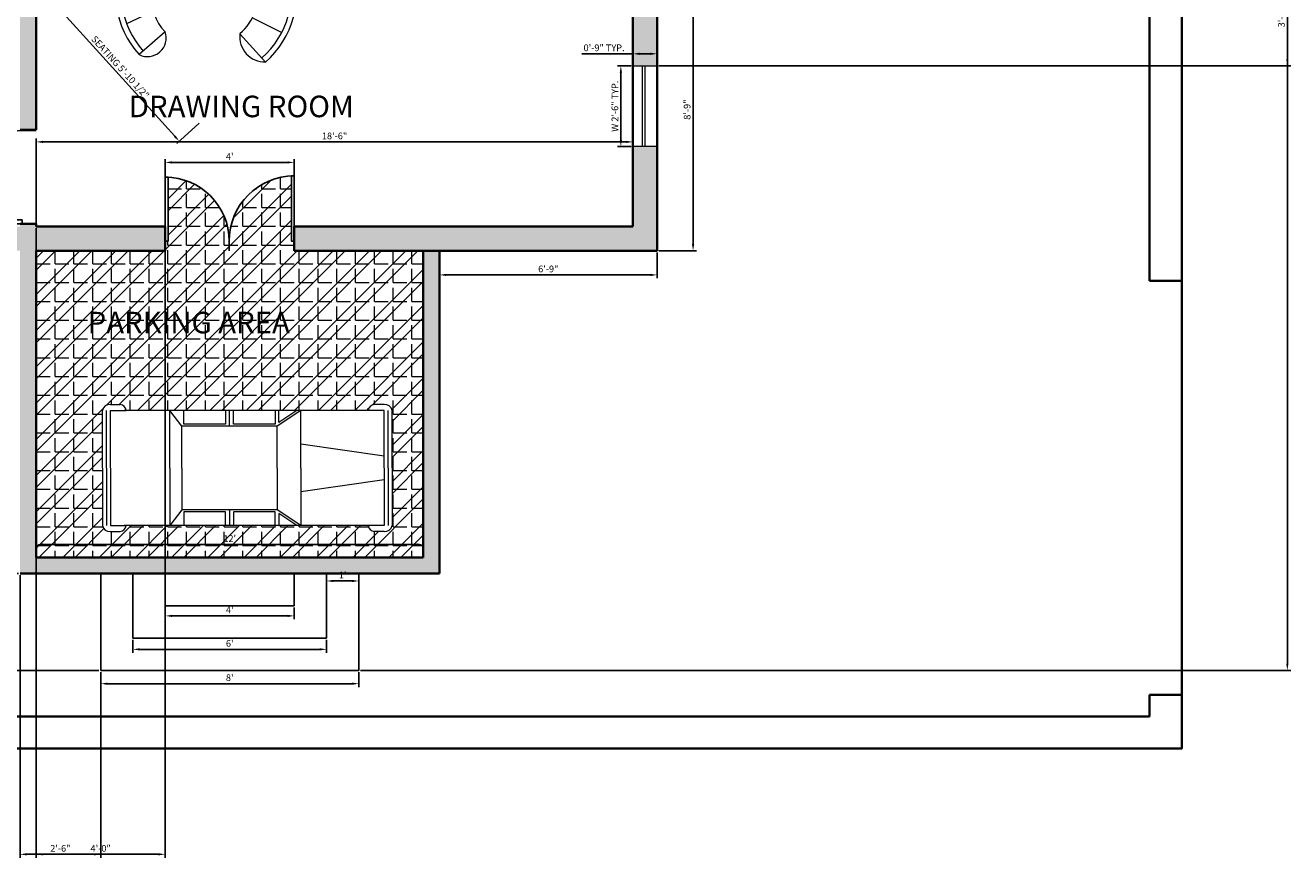
# Model space of a CAD drawing. Units: inches. Extents: x 2901 to 5923, y 918 to 2827.
# Tile 9 of 16: x 4585 to 5056, y 918 to 1227. Entities that reach past the tile are written whole.
import ezdxf

# ---------------------------------------------------------------- set-up
doc = ezdxf.new("R2010")
doc.units = ezdxf.units.IN
for name, color, linetype, lineweight in [('A-ANNO-DIMS', 2, 'Continuous', 18), ('A-AREA-IDEN', 7, 'Continuous', 25), ('A-EQPM-VEHI', 8, 'Continuous', 18), ('A-FLOR-PATT', 252, 'Continuous', 13), ('A-FLOR-STRS', 7, 'Continuous', 25), ('A-GLAZ', 4, 'Continuous', 18), ('A-WALL-PATT', 7, 'Continuous', 13), ('C-PROP', 7, 'Continuous', 35), ('doors', 240, 'Continuous', 25), ('furniture', 160, 'Continuous', 18), ('walls', 7, 'Continuous', 35)]:
    doc.layers.add(name, color=color, linetype=linetype, lineweight=lineweight)
doc.styles.get("Standard").update_dxf_attribs({"font": 'arial.ttf'})
doc.dimstyles.new('Copy of ISO-25', dxfattribs={"dimtxt": 2.5, "dimasz": 2.5, "dimexe": 1.25, "dimexo": 0.625, "dimtad": 1, "dimdec": 1, "dimlunit": 4, "dimtxsty": 'Standard', "dimcen": 2.5, "dimadec": 0, "dimazin": 0, "dimtfac": 1, "dimtdec": 1, "dimtmove": 0, "dimatfit": 3, "dimfxl": 1, "dimarcsym": 0})

# ---------------------------------------------------------------- blocks, each defined once
blk = doc.blocks.new('*U8')
for p, q in [((0, 0), (0, -6)), ((-40, 0), (-40, -6))]:
    blk.add_line(p, q)
blk.add_lwpolyline([(0, 0), (0, 40), (-1.75, 40), (-1.75, 0)], close=True)
blk.add_arc((0, 0), 40, 90, 180)
blk = doc.blocks.new('*U6')
for p, q in [((0, 0), (0, -6)), ((40, 0), (40, -6))]:
    blk.add_line(p, q)
blk.add_lwpolyline([(0, 0), (0, 40), (1.75, 40), (1.75, 0)], close=True)
blk.add_arc((0, 0), 40, 0, 90)
blk = doc.blocks.new('*U2')
for p, q in [((0, 0), (0, -6)), ((40, 0), (40, -6))]:
    blk.add_line(p, q)
blk.add_lwpolyline([(0, 0), (0, 40), (1.75, 40), (1.75, 0)], close=True)
blk.add_arc((0, 0), 40, 0, 90)
blk = doc.blocks.new('A$C0ECE726C')
for p, q in [((1694, 2620), (1694, 3331)), ((1322, 2571), (1110, 3122)), ((1023, 2382), (606, 2799)), ((787, 2067), (221, 2311)), ((701, 1673), (142, 1666)), ((2687, 1673), (3320, 1664)), ((795, 1248), (221, 1075)), ((2593, 1248), (3113, 1091)), ((1016, 941), (551, 587)), ((2372, 941), (2811, 607)), ((1315, 753), (1055, 225)), ((1694, 100), (1694, 697)), ((2073, 753), (2322, 247))]:
    blk.add_line(p, q)
blk.add_circle((1652, 1618), 420)
for centre, radius, start, end in [((1660, 1660), 1660, 88.7606, 0.1441), ((1392, 2970), 462, 310.7368, 49.2632), ((1660, 1660), 1560, 88.7606, 0.2051), ((1660, 1660), 960, 87.986, 272.014), ((3002, 1543), 340, 20.831, 157.5545), ((1728, 1660), 960, 267.986, 0.781)]:
    blk.add_arc(centre, radius, start, end)
blk = doc.blocks.new('*U22')
for p, q in [((3, -10), (3, 974)), ((70, -10), (70, 973)), ((138, 1075), (308, 1075)), ((138, 973), (410, 973)), ((138, -10), (138, 971)), ((410, 973), (4581, 973)), ((1563, -10), (1563, 973)), ((1563, 973), (1969, 702)), ((1630, 973), (1936, 769)), ((1936, 769), (1936, 973)), ((2003, 973), (2003, 736)), ((2716, 736), (2716, 973)), ((2783, 702), (2783, 973)), ((2851, 973), (2851, 736)), ((3563, 736), (3563, 973)), ((3597, 702), (3801, 973)), ((3801, -10), (3801, 973)), ((4818, 973), (4547, 973)), ((4818, 1075), (4649, 1075)), ((4818, -10), (4818, 971)), ((4886, -10), (4886, 973)), ((4954, -10), (4954, 974)), ((1969, 702), (3597, 702)), ((1969, -10), (1969, 702)), ((2003, 736), (2716, 736)), ((2851, 736), (3563, 736)), ((3597, -10), (3597, 702)), ((138, 193), (1563, 396)), ((3, -11), (3, -995)), ((70, -10), (70, -994)), ((138, -11), (138, -992)), ((138, -214), (1563, -417)), ((1563, -10), (1563, -994)), ((1969, -10), (1969, -723)), ((3597, -10), (3597, -723)), ((3801, -10), (3801, -994)), ((4818, -11), (4818, -992)), ((4886, -10), (4886, -994)), ((4954, -11), (4954, -995)), ((1563, -994), (1969, -723)), ((1630, -994), (1936, -790)), ((1936, -790), (1936, -994)), ((1969, -723), (3597, -723)), ((2003, -994), (2003, -757)), ((2003, -757), (2716, -757)), ((2716, -757), (2716, -994)), ((2783, -723), (2783, -994)), ((2851, -757), (3563, -757)), ((2851, -994), (2851, -757)), ((3563, -757), (3563, -994)), ((3597, -723), (3801, -994)), ((138, -994), (410, -994)), ((410, -994), (4581, -994)), ((4818, -994), (4547, -994)), ((138, -1096), (308, -1096)), ((4818, -1096), (4649, -1096))]:
    blk.add_line(p, q)
for centre, radius, start, end in [((128, 946), 129, 85.6455, 168.0943), ((291, 956), 120, 8.1301, 81.87), ((4665, 956), 120, 98.13, 171.8699), ((4828, 946), 129, 11.9057, 94.3545), ((128, -967), 129, 191.9057, 274.3545), ((291, -977), 120, 278.13, 351.8699), ((4665, -977), 120, 188.1301, 261.87), ((4828, -967), 129, 265.6455, 348.0943)]:
    blk.add_arc(centre, radius, start, end)
blk = doc.blocks.new('*D32')
at = {"layer": 'A-ANNO-DIMS', "color": 0, "lineweight": -2, "transparency": 16777216}
for p, q in [((4589.07, 1030.02), (4589.07, 1035.46)), ((4591.57, 1034.21), (4730.57, 1034.21)), ((4733.07, 1030.02), (4733.07, 1035.46))]:
    blk.add_line(p, q, dxfattribs=at)
at = {"layer": 'A-ANNO-DIMS', "color": 0, "transparency": 16777216}
for points in [[(4591.57, 1034.63), (4591.57, 1033.8), (4589.07, 1034.21)], [(4730.57, 1034.63), (4730.57, 1033.8), (4733.07, 1034.21)]]:
    blk.add_solid(points, dxfattribs=at)
at = {"layer": 'Defpoints', "color": 0, "transparency": 16777216}
for p in [(4733.07, 1034.21), (4589.07, 1029.4), (4733.07, 1029.4)]:
    blk.add_point(p, dxfattribs=at)
at = {"layer": 'A-ANNO-DIMS', "color": 0, "transparency": 16777216, "insert": (4661.07, 1036.09), "char_height": 2.5, "attachment_point": 5}
blk.add_mtext("12'", dxfattribs=at)
blk = doc.blocks.new('*D33')
at = {"layer": 'A-ANNO-DIMS', "color": 0, "lineweight": -2, "transparency": 16777216}
for p, q in [((4739.07, 1142.77), (4739.07, 1133.19)), ((4820.07, 1142.77), (4820.07, 1133.19)), ((4741.57, 1134.44), (4817.57, 1134.44))]:
    blk.add_line(p, q, dxfattribs=at)
at = {"layer": 'A-ANNO-DIMS', "color": 0, "transparency": 16777216}
for points in [[(4741.57, 1134.86), (4741.57, 1134.02), (4739.07, 1134.44)], [(4817.57, 1134.86), (4817.57, 1134.02), (4820.07, 1134.44)]]:
    blk.add_solid(points, dxfattribs=at)
at = {"layer": 'Defpoints', "color": 0, "transparency": 16777216}
for p in [(4739.07, 1143.4), (4820.07, 1143.4), (4820.07, 1134.44)]:
    blk.add_point(p, dxfattribs=at)
at = {"layer": 'A-ANNO-DIMS', "color": 0, "transparency": 16777216, "insert": (4779.57, 1136.34), "char_height": 2.5, "attachment_point": 5}
blk.add_mtext('6\'-9"', dxfattribs=at)
blk = doc.blocks.new('*D34')
at = {"layer": 'A-ANNO-DIMS', "color": 0, "lineweight": -2, "transparency": 16777216}
for p, q in [((4820.69, 1248.4), (4834.68, 1248.4)), ((4833.43, 1145.9), (4833.43, 1245.9)), ((4820.69, 1143.4), (4834.68, 1143.4))]:
    blk.add_line(p, q, dxfattribs=at)
at = {"layer": 'A-ANNO-DIMS', "color": 0, "transparency": 16777216}
for points in [[(4833.01, 1245.9), (4833.85, 1245.9), (4833.43, 1248.4)], [(4833.01, 1145.9), (4833.85, 1145.9), (4833.43, 1143.4)]]:
    blk.add_solid(points, dxfattribs=at)
at = {"layer": 'Defpoints', "color": 0, "transparency": 16777216}
for p in [(4820.07, 1248.4), (4833.43, 1248.4), (4820.07, 1143.4)]:
    blk.add_point(p, dxfattribs=at)
at = {"layer": 'A-ANNO-DIMS', "color": 0, "transparency": 16777216, "insert": (4831.53, 1195.9), "char_height": 2.5, "attachment_point": 5, "rotation": 90}
blk.add_mtext('8\'-9"', dxfattribs=at)
blk = doc.blocks.new('*D51')
at = {"layer": 'A-ANNO-DIMS', "color": 0, "lineweight": -2, "transparency": 16777216}
for p, q in [((4613.07, 986.77), (4613.07, 981.19)), ((4709.07, 986.77), (4709.07, 981.19)), ((4615.57, 982.44), (4706.57, 982.44))]:
    blk.add_line(p, q, dxfattribs=at)
at = {"layer": 'A-ANNO-DIMS', "color": 0, "transparency": 16777216}
for points in [[(4615.57, 982.85), (4615.57, 982.02), (4613.07, 982.44)], [(4706.57, 982.85), (4706.57, 982.02), (4709.07, 982.44)]]:
    blk.add_solid(points, dxfattribs=at)
at = {"layer": 'Defpoints', "color": 0, "transparency": 16777216}
for p in [(4613.07, 987.4), (4709.07, 987.4), (4709.07, 982.44)]:
    blk.add_point(p, dxfattribs=at)
at = {"layer": 'A-ANNO-DIMS', "color": 0, "transparency": 16777216, "insert": (4661.07, 984.34), "char_height": 2.5, "attachment_point": 5}
blk.add_mtext("8'", dxfattribs=at)
blk = doc.blocks.new('*D52')
at = {"layer": 'A-ANNO-DIMS', "color": 0, "lineweight": -2, "transparency": 16777216}
for p, q in [((4625.07, 998.77), (4625.07, 993.96)), ((4697.07, 998.77), (4697.07, 993.96)), ((4627.57, 995.21), (4694.57, 995.21))]:
    blk.add_line(p, q, dxfattribs=at)
at = {"layer": 'A-ANNO-DIMS', "color": 0, "transparency": 16777216}
for points in [[(4627.57, 995.62), (4627.57, 994.79), (4625.07, 995.21)], [(4694.57, 995.62), (4694.57, 994.79), (4697.07, 995.21)]]:
    blk.add_solid(points, dxfattribs=at)
at = {"layer": 'Defpoints', "color": 0, "transparency": 16777216}
for p in [(4625.07, 999.4), (4697.07, 999.4), (4697.07, 995.21)]:
    blk.add_point(p, dxfattribs=at)
at = {"layer": 'A-ANNO-DIMS', "color": 0, "transparency": 16777216, "insert": (4661.07, 997.11), "char_height": 2.5, "attachment_point": 5}
blk.add_mtext("6'", dxfattribs=at)
blk = doc.blocks.new('*D53')
at = {"layer": 'A-ANNO-DIMS', "color": 0, "lineweight": -2, "transparency": 16777216}
for p, q in [((4637.07, 1010.77), (4637.07, 1006.4)), ((4639.57, 1007.65), (4682.57, 1007.65)), ((4685.07, 1010.77), (4685.07, 1006.4))]:
    blk.add_line(p, q, dxfattribs=at)
at = {"layer": 'A-ANNO-DIMS', "color": 0, "transparency": 16777216}
for points in [[(4639.57, 1008.07), (4639.57, 1007.24), (4637.07, 1007.65)], [(4682.57, 1008.07), (4682.57, 1007.24), (4685.07, 1007.65)]]:
    blk.add_solid(points, dxfattribs=at)
at = {"layer": 'Defpoints', "color": 0, "transparency": 16777216}
for p in [(4637.07, 1011.4), (4685.07, 1011.4), (4685.07, 1007.65)]:
    blk.add_point(p, dxfattribs=at)
at = {"layer": 'A-ANNO-DIMS', "color": 0, "transparency": 16777216, "insert": (4661.07, 1009.53), "char_height": 2.5, "attachment_point": 5}
blk.add_mtext("4'", dxfattribs=at)
blk = doc.blocks.new('*D54')
at = {"layer": 'A-ANNO-DIMS', "color": 0, "lineweight": -2, "transparency": 16777216}
for p, q in [((4697.07, 1022.77), (4697.07, 1019.39)), ((4709.07, 1022.77), (4709.07, 1019.39)), ((4699.57, 1020.64), (4706.57, 1020.64))]:
    blk.add_line(p, q, dxfattribs=at)
at = {"layer": 'A-ANNO-DIMS', "color": 0, "transparency": 16777216}
for points in [[(4699.57, 1021.05), (4699.57, 1020.22), (4697.07, 1020.64)], [(4706.57, 1021.05), (4706.57, 1020.22), (4709.07, 1020.64)]]:
    blk.add_solid(points, dxfattribs=at)
at = {"layer": 'Defpoints', "color": 0, "transparency": 16777216}
for p in [(4697.07, 1023.4), (4709.07, 1023.4), (4709.07, 1020.64)]:
    blk.add_point(p, dxfattribs=at)
at = {"layer": 'A-ANNO-DIMS', "color": 0, "transparency": 16777216, "insert": (4703.07, 1022.52), "char_height": 2.5, "attachment_point": 5}
blk.add_mtext("1'", dxfattribs=at)
blk = doc.blocks.new('*D59')
at = {"layer": 'A-ANNO-DIMS', "color": 0, "lineweight": -2, "transparency": 16777216}
for p, q in [((4637.07, 1153.02), (4637.07, 1177.52)), ((4685.07, 1153.02), (4685.07, 1177.52)), ((4639.57, 1176.27), (4682.57, 1176.27))]:
    blk.add_line(p, q, dxfattribs=at)
at = {"layer": 'A-ANNO-DIMS', "color": 0, "transparency": 16777216}
for points in [[(4639.57, 1176.68), (4639.57, 1175.85), (4637.07, 1176.27)], [(4682.57, 1176.68), (4682.57, 1175.85), (4685.07, 1176.27)]]:
    blk.add_solid(points, dxfattribs=at)
at = {"layer": 'Defpoints', "color": 0, "transparency": 16777216}
for p in [(4685.07, 1176.27), (4637.07, 1152.4), (4685.07, 1152.4)]:
    blk.add_point(p, dxfattribs=at)
at = {"layer": 'A-ANNO-DIMS', "color": 0, "transparency": 16777216, "insert": (4661.07, 1178.14), "char_height": 2.5, "attachment_point": 5}
blk.add_mtext("4'", dxfattribs=at)
blk = doc.blocks.new('*D61')
at = {"layer": 'A-ANNO-DIMS', "color": 0, "lineweight": -2, "transparency": 16777216}
for p, q in [((4589.07, 1153.02), (4589.07, 1185.15)), ((4591.57, 1183.9), (4808.57, 1183.9)), ((4811.07, 1153.02), (4811.07, 1185.15))]:
    blk.add_line(p, q, dxfattribs=at)
at = {"layer": 'A-ANNO-DIMS', "color": 0, "transparency": 16777216}
for points in [[(4591.57, 1184.32), (4591.57, 1183.49), (4589.07, 1183.9)], [(4808.57, 1184.32), (4808.57, 1183.49), (4811.07, 1183.9)]]:
    blk.add_solid(points, dxfattribs=at)
at = {"layer": 'Defpoints', "color": 0, "transparency": 16777216}
for p in [(4811.07, 1183.9), (4589.07, 1152.4), (4811.07, 1152.4)]:
    blk.add_point(p, dxfattribs=at)
at = {"layer": 'A-ANNO-DIMS', "color": 0, "transparency": 16777216, "insert": (4700.07, 1185.8), "char_height": 2.5, "attachment_point": 5}
blk.add_mtext('18\'-6"', dxfattribs=at)
blk = doc.blocks.new('WIN-30')
for p, q in [((0, 30), (9, 30)), ((4.5, 30), (4.5, 0)), ((5.5, 30), (5.5, 0)), ((9, 30), (9, 0)), ((9, 0), (0, 0))]:
    blk.add_line(p, q)
blk = doc.blocks.new('*D77')
at = {"layer": 'A-ANNO-DIMS', "color": 0, "lineweight": -2, "transparency": 16777216}
for p, q in [((4810.44, 1212.16), (4805.32, 1212.16)), ((4806.57, 1209.66), (4806.57, 1184.66)), ((4810.44, 1182.16), (4805.32, 1182.16))]:
    blk.add_line(p, q, dxfattribs=at)
at = {"layer": 'A-ANNO-DIMS', "color": 0, "transparency": 16777216}
for points in [[(4806.15, 1209.66), (4806.99, 1209.66), (4806.57, 1212.16)], [(4806.15, 1184.66), (4806.99, 1184.66), (4806.57, 1182.16)]]:
    blk.add_solid(points, dxfattribs=at)
at = {"layer": 'Defpoints', "color": 0, "transparency": 16777216}
for p in [(4811.07, 1212.16), (4806.57, 1182.16), (4811.07, 1182.16)]:
    blk.add_point(p, dxfattribs=at)
at = {"layer": 'A-ANNO-DIMS', "color": 0, "transparency": 16777216, "insert": (4804.67, 1197.16), "char_height": 2.5, "attachment_point": 5, "rotation": 90}
blk.add_mtext('W 2\'-6" TYP.', dxfattribs=at)
blk = doc.blocks.new('*D78')
at = {"layer": 'A-ANNO-DIMS', "color": 0, "lineweight": -2, "transparency": 16777216}
for p, q in [((4811.07, 1216.66), (4792.08, 1216.66)), ((4811.07, 1212.79), (4811.07, 1217.91)), ((4817.57, 1216.66), (4813.57, 1216.66)), ((4820.07, 1212.79), (4820.07, 1217.91))]:
    blk.add_line(p, q, dxfattribs=at)
at = {"layer": 'A-ANNO-DIMS', "color": 0, "transparency": 16777216}
for points in [[(4813.57, 1217.08), (4813.57, 1216.24), (4811.07, 1216.66)], [(4817.57, 1217.08), (4817.57, 1216.24), (4820.07, 1216.66)]]:
    blk.add_solid(points, dxfattribs=at)
at = {"layer": 'Defpoints', "color": 0, "transparency": 16777216}
for p in [(4811.07, 1216.66), (4811.07, 1212.16), (4820.07, 1212.16)]:
    blk.add_point(p, dxfattribs=at)
at = {"layer": 'A-ANNO-DIMS', "color": 0, "transparency": 16777216, "insert": (4800.32, 1218.56), "char_height": 2.5, "attachment_point": 5}
blk.add_mtext('0\'-9" TYP.', dxfattribs=at)
blk = doc.blocks.new('*D85')
at = {"layer": 'A-ANNO-DIMS', "color": 0, "lineweight": -2, "transparency": 16777216}
for p, q in [((4602.46, 1242.89), (4594.18, 1235.39)), ((4596.79, 1234.37), (4640.62, 1186)), ((4649.65, 1190.81), (4641.38, 1183.31))]:
    blk.add_line(p, q, dxfattribs=at)
at = {"layer": 'A-ANNO-DIMS', "color": 0, "transparency": 16777216}
for points in [[(4597.1, 1234.65), (4596.48, 1234.09), (4595.11, 1236.23)], [(4640.93, 1186.28), (4640.32, 1185.72), (4642.3, 1184.15)]]:
    blk.add_solid(points, dxfattribs=at)
at = {"layer": 'Defpoints', "color": 0, "transparency": 16777216}
for p in [(4602.92, 1243.31), (4650.11, 1191.23), (4642.3, 1184.15)]:
    blk.add_point(p, dxfattribs=at)
at = {"layer": 'A-ANNO-DIMS', "color": 0, "transparency": 16777216, "insert": (4620.13, 1211.48), "char_height": 2.5, "attachment_point": 5, "rotation": 312.1851}
blk.add_mtext('SEATING 5\'-10 1/2"', dxfattribs=at)
blk = doc.blocks.new('*D89')
at = {"layer": 'A-ANNO-DIMS', "color": 0, "lineweight": -2, "transparency": 16777216}
for p, q in [((4892.69, 1630.4), (5055.73, 1630.4)), ((5054.48, 989.9), (5054.48, 1627.9)), ((4709.69, 987.4), (5055.73, 987.4))]:
    blk.add_line(p, q, dxfattribs=at)
at = {"layer": 'A-ANNO-DIMS', "color": 0, "transparency": 16777216}
for points in [[(5054.06, 1627.9), (5054.9, 1627.9), (5054.48, 1630.4)], [(5054.06, 989.9), (5054.9, 989.9), (5054.48, 987.4)]]:
    blk.add_solid(points, dxfattribs=at)
at = {"layer": 'Defpoints', "color": 0, "transparency": 16777216}
for p in [(4892.07, 1630.4), (5054.48, 1630.4), (4709.07, 987.4)]:
    blk.add_point(p, dxfattribs=at)
at = {"layer": 'A-ANNO-DIMS', "color": 0, "transparency": 16777216, "insert": (5052.58, 1308.9), "char_height": 2.5, "attachment_point": 5, "rotation": 90}
blk.add_mtext('53\'-7"', dxfattribs=at)
blk = doc.blocks.new('*D99')
at = {"layer": 'A-ANNO-DIMS', "color": 0, "lineweight": -2, "transparency": 16777216}
for p, q in [((4820.69, 1248.4), (5055.73, 1248.4)), ((5054.48, 1214.66), (5054.48, 1245.9)), ((4820.69, 1212.16), (5055.73, 1212.16))]:
    blk.add_line(p, q, dxfattribs=at)
at = {"layer": 'A-ANNO-DIMS', "color": 0, "transparency": 16777216}
for points in [[(5054.06, 1245.9), (5054.9, 1245.9), (5054.48, 1248.4)], [(5054.06, 1214.66), (5054.9, 1214.66), (5054.48, 1212.16)]]:
    blk.add_solid(points, dxfattribs=at)
at = {"layer": 'Defpoints', "color": 0, "transparency": 16777216}
for p in [(4820.07, 1248.4), (5054.48, 1248.4), (4820.07, 1212.16)]:
    blk.add_point(p, dxfattribs=at)
at = {"layer": 'A-ANNO-DIMS', "color": 0, "transparency": 16777216, "insert": (5052.58, 1230.28), "char_height": 2.5, "attachment_point": 5, "rotation": 90}
blk.add_mtext('3\'-0"', dxfattribs=at)
blk = doc.blocks.new('*D100')
at = {"layer": 'A-ANNO-DIMS', "color": 0, "lineweight": -2, "transparency": 16777216}
for p, q in [((4589.07, 1151.77), (4589.07, 917.74)), ((4637.07, 1151.77), (4637.07, 917.74)), ((4591.57, 918.99), (4634.57, 918.99))]:
    blk.add_line(p, q, dxfattribs=at)
at = {"layer": 'A-ANNO-DIMS', "color": 0, "transparency": 16777216}
for points in [[(4591.57, 919.41), (4591.57, 918.58), (4589.07, 918.99)], [(4634.57, 919.41), (4634.57, 918.58), (4637.07, 918.99)]]:
    blk.add_solid(points, dxfattribs=at)
at = {"layer": 'Defpoints', "color": 0, "transparency": 16777216}
for p in [(4589.07, 1152.4), (4637.07, 1152.4), (4637.07, 918.99)]:
    blk.add_point(p, dxfattribs=at)
at = {"layer": 'A-ANNO-DIMS', "color": 0, "transparency": 16777216, "insert": (4613.07, 920.89), "char_height": 2.5, "attachment_point": 5}
blk.add_mtext('4\'-0"', dxfattribs=at)
blk = doc.blocks.new('*D103')
at = {"layer": 'A-ANNO-DIMS', "color": 0, "lineweight": -2, "transparency": 16777216}
for p, q in [((4583.07, 1022.77), (4583.07, 917.74)), ((4613.07, 986.77), (4613.07, 917.74)), ((4585.57, 918.99), (4610.57, 918.99))]:
    blk.add_line(p, q, dxfattribs=at)
at = {"layer": 'A-ANNO-DIMS', "color": 0, "transparency": 16777216}
for points in [[(4585.57, 919.41), (4585.57, 918.58), (4583.07, 918.99)], [(4610.57, 919.41), (4610.57, 918.58), (4613.07, 918.99)]]:
    blk.add_solid(points, dxfattribs=at)
at = {"layer": 'Defpoints', "color": 0, "transparency": 16777216}
for p in [(4583.07, 1023.4), (4613.07, 987.4), (4613.07, 918.99)]:
    blk.add_point(p, dxfattribs=at)
at = {"layer": 'A-ANNO-DIMS', "color": 0, "transparency": 16777216, "insert": (4598.07, 920.89), "char_height": 2.5, "attachment_point": 5}
blk.add_mtext('2\'-6"', dxfattribs=at)
blk = doc.blocks.new('*D104')
at = {"layer": 'A-ANNO-DIMS', "color": 0, "lineweight": -2, "transparency": 16777216}
for p, q in [((4582.44, 1023.4), (4247.63, 1023.4)), ((4248.88, 1020.9), (4248.88, 989.9)), ((4612.44, 987.4), (4247.63, 987.4))]:
    blk.add_line(p, q, dxfattribs=at)
at = {"layer": 'A-ANNO-DIMS', "color": 0, "transparency": 16777216}
for points in [[(4248.46, 1020.9), (4249.3, 1020.9), (4248.88, 1023.4)], [(4248.46, 989.9), (4249.3, 989.9), (4248.88, 987.4)]]:
    blk.add_solid(points, dxfattribs=at)
at = {"layer": 'Defpoints', "color": 0, "transparency": 16777216}
for p in [(4583.07, 1023.4), (4248.88, 987.4), (4613.07, 987.4)]:
    blk.add_point(p, dxfattribs=at)
at = {"layer": 'A-ANNO-DIMS', "color": 0, "transparency": 16777216, "insert": (4246.98, 1005.4), "char_height": 2.5, "attachment_point": 5, "rotation": 90}
blk.add_mtext('3\'-0"', dxfattribs=at)

msp = doc.modelspace()

# ---------------------------------------------------------------- hatches: boundary and pattern name
at = {"layer": 'A-FLOR-PATT'}
h = msp.add_hatch(dxfattribs=at)
h.set_pattern_fill('ANSI32', color=256)
h.paths.add_polyline_path([(4883.07, 1621.4), (4739.07, 1621.4), (4739.07, 1564.39, -0.396616), (4774.43, 1529.97), (4774.46, 1529.97), (4774.46, 1528.4), (4883.07, 1528.4)])
h.paths.add_polyline_path([(4733.07, 1143.4), (4685.07, 1143.4), (4685.07, 1147.03), (4684.01, 1147.03), (4684.01, 1171.22, 0.413071), (4660.87, 1146.06, 0.412532), (4638.11, 1170.77), (4638.11, 1146.97), (4637.07, 1143.4), (4589.07, 1143.4), (4589.07, 1029.4), (4733.07, 1029.4)])
h.paths.add_polyline_path([(4620.35, 1086.26, -0.333335), (4622.56, 1084.04), (4622.56, 1084.04), (4712.62, 1084.04, -0.333335), (4714.84, 1086.26), (4718.53, 1086.26, -0.376086), (4721.48, 1084.04), (4721.48, 1062.64), (4721.48, 1041.23, -0.333387), (4718.96, 1039.01), (4714.84, 1039.01, -0.333335), (4712.62, 1041.23), (4712.62, 1041.23), (4622.56, 1041.23, -0.333335), (4620.35, 1039.01), (4616.66, 1039.01, -0.376086), (4613.71, 1041.23), (4613.71, 1062.63), (4613.71, 1084.04, -0.333387), (4616.23, 1086.26)], flags=16)
h.paths.add_polyline_path([(4638.8, 1084.04), (4643.23, 1078.14), (4678.67, 1078.14), (4687.53, 1084.04), (4687.53, 1071.49), (4718.53, 1067.06), (4718.53, 1062.64), (4718.53, 1058.21), (4687.53, 1053.78), (4687.53, 1041.23), (4678.67, 1047.13), (4643.23, 1047.13), (4638.8, 1041.23), (4638.8, 1062.63)], flags=0)
h = msp.add_hatch(dxfattribs=at)
h.set_pattern_fill('ANGLE', color=256)
h.set_pattern_definition([(0, (0, 0), (0, 6.985), [5.08, -1.905]), (90, (0, 0), (-6.985, 4e-16), [5.08, -1.905])])
h.paths.add_polyline_path([(4733.07, 1143.4), (4685.07, 1143.4), (4685.07, 1147.03), (4684.01, 1147.03), (4684.01, 1171.22, 0.413071), (4660.87, 1146.06, 0.412532), (4638.11, 1170.77), (4638.11, 1146.97), (4637.07, 1143.4), (4589.07, 1143.4), (4589.07, 1029.4), (4733.07, 1029.4)])
h.paths.add_polyline_path([(4712.62, 1084.04, -0.333335), (4714.84, 1086.26), (4718.53, 1086.26, -0.376086), (4721.48, 1084.04), (4721.48, 1062.64), (4721.48, 1041.23, -0.333387), (4718.96, 1039.01), (4714.84, 1039.01, -0.333335), (4712.62, 1041.23), (4712.62, 1041.23), (4622.56, 1041.23, -0.333335), (4620.35, 1039.01), (4616.66, 1039.01, -0.376086), (4613.71, 1041.23), (4613.71, 1062.63), (4613.71, 1084.04, -0.333387), (4616.23, 1086.26), (4620.35, 1086.26, -0.333335), (4622.56, 1084.04), (4622.56, 1084.04)], flags=16)
h.paths.add_polyline_path([(4687.53, 1084.04), (4687.53, 1071.49), (4718.53, 1067.06), (4718.53, 1062.64), (4718.53, 1058.21), (4687.53, 1053.78), (4687.53, 1041.23), (4678.67, 1047.13), (4643.23, 1047.13), (4638.8, 1041.23), (4638.8, 1062.63), (4638.8, 1084.04), (4643.23, 1078.14), (4678.67, 1078.14)], flags=0)
at = {"layer": 'A-WALL-PATT'}
h = msp.add_hatch(color=256, dxfattribs=at)
h.dxf.hatch_style = 1
h.paths.add_polyline_path([(4439.07, 1447.4), (4583.07, 1447.4), (4583.07, 1340.4), (4589.07, 1340.4), (4589.07, 1453.4), (4589.07, 1455.39), (4583.07, 1455.39), (4583.07, 1453.4), (4439.07, 1453.4), (4439.07, 1501.84), (4430.07, 1501.84), (4430.07, 1399.4), (4439.07, 1399.4)])
h.paths.add_polyline_path([(4439.07, 1621.4), (4487.07, 1621.4), (4487.07, 1630.4), (4430.07, 1630.4), (4430.07, 1561.84), (4439.07, 1561.84)])
h.paths.add_polyline_path([(4630.61, 1630.4), (4535.07, 1630.4), (4535.07, 1621.4), (4583.07, 1621.4), (4583.07, 1495.4), (4589.07, 1495.4), (4637.07, 1495.4), (4637.07, 1501.4), (4589.07, 1501.4), (4589.07, 1621.4), (4630.61, 1621.4)])
h.paths.add_polyline_path([(4892.07, 1630.4), (4690.61, 1630.4), (4690.61, 1621.4), (4733.07, 1621.4), (4733.07, 1564.4), (4739.07, 1564.4), (4739.07, 1621.4), (4883.07, 1621.4), (4883.07, 1528.4), (4739.07, 1528.4), (4733.07, 1528.4), (4733.07, 1501.4), (4685.07, 1501.4), (4685.07, 1495.4), (4739.07, 1495.4), (4739.07, 1519.4), (4787.07, 1519.4), (4787.07, 1423.4), (4739.07, 1423.4), (4739.07, 1456.67), (4733.07, 1456.67), (4733.07, 1340.4), (4739.07, 1340.4), (4739.07, 1417.4), (4787.07, 1417.4), (4793.07, 1417.4), (4793.07, 1423.4), (4793.07, 1519.4), (4883.07, 1519.4), (4883.07, 1482.87), (4892.07, 1482.87)])
h.paths.add_polyline_path([(4892.07, 1458.87), (4883.07, 1458.87), (4883.07, 1423.4), (4823.07, 1423.4), (4823.07, 1417.4), (4883.07, 1417.4), (4883.07, 1363.31), (4892.07, 1363.31)], flags=17)
h.paths.add_polyline_path([(4892.07, 1303.31), (4883.07, 1303.31), (4883.07, 1255.4), (4739.07, 1255.4), (4739.07, 1304.4), (4733.07, 1304.4), (4733.07, 1303.4), (4733.07, 1297.4), (4733.07, 1255.4), (4733.07, 1248.4), (4811.07, 1248.4), (4811.07, 1212.16), (4820.07, 1212.16), (4820.07, 1248.4), (4892.07, 1248.4)])
h.paths.add_polyline_path([(4820.07, 1182.16), (4811.07, 1182.16), (4811.07, 1152.4), (4685.07, 1152.4), (4685.07, 1147.03), (4685.07, 1143.4), (4733.07, 1143.4), (4811.07, 1143.4), (4814.07, 1143.4), (4820.07, 1143.4)])
h.paths.add_polyline_path([(4637.07, 1152.4), (4589.07, 1152.4), (4589.07, 1153.4), (4583.86, 1153.4), (4583.07, 1153.4), (4583.07, 1152.4), (4511.07, 1152.4), (4511.07, 1182.16), (4502.07, 1182.16), (4502.07, 1143.4), (4568.07, 1143.4), (4583.07, 1143.4), (4583.07, 1023.4), (4739.07, 1023.4), (4739.07, 1143.4), (4733.07, 1143.4), (4733.07, 1029.4), (4589.07, 1029.4), (4589.07, 1143.4), (4637.07, 1143.4), (4637.07, 1146.97)])
h.paths.add_polyline_path([(4511.07, 1246.4), (4583.07, 1246.4), (4583.07, 1188.4), (4589.07, 1188.4), (4589.07, 1246.4), (4589.07, 1248.4), (4589.07, 1255.4), (4589.07, 1297.4), (4697.07, 1297.4), (4697.07, 1303.4), (4589.07, 1303.4), (4589.07, 1304.4), (4583.07, 1304.4), (4583.07, 1255.4), (4439.07, 1255.4), (4439.07, 1261.4), (4439.07, 1351.4), (4430.07, 1351.4), (4430.07, 1252.4), (4430.07, 1246.4), (4439.07, 1246.4), (4487.07, 1246.4), (4502.07, 1246.4), (4502.07, 1212.16), (4511.07, 1212.16)])

# ---------------------------------------------------------------- linework, layer by layer
at = {"layer": 'A-FLOR-STRS'}
for p, q in [((4625.07, 1023.4), (4613.07, 1023.4)), ((4613.07, 1023.4), (4613.07, 987.4)), ((4625.07, 999.4), (4625.07, 1023.4)), ((4637.07, 1023.4), (4637.07, 1011.4)), ((4685.07, 1011.4), (4685.07, 1023.4)), ((4685.07, 1023.4), (4697.07, 1023.4)), ((4697.07, 1023.4), (4697.07, 1011.4)), ((4709.07, 987.4), (4709.07, 1023.4)), ((4637.07, 1011.4), (4685.07, 1011.4)), ((4697.07, 1011.4), (4697.07, 999.4)), ((4637.07, 999.4), (4625.07, 999.4)), ((4697.07, 999.4), (4637.07, 999.4)), ((4613.07, 987.4), (4709.07, 987.4))]:
    msp.add_line(p, q, dxfattribs=at)
at = {"layer": 'A-GLAZ'}
msp.add_line((4820.07, 1212.16), (4820.07, 1182.16), dxfattribs=at)
at = {"layer": 'C-PROP'}
for p, q in [((5015.18, 1143.4), (5015.18, 978.26)), ((5003.18, 1132.27), (5015.18, 1132.27)), ((5015.18, 978.26), (5003.18, 978.26))]:
    msp.add_line(p, q, dxfattribs=at)
msp.add_lwpolyline([(4288.18, 1684.29), (5015.18, 1684.29), (5015.18, 958.29), (4288.18, 958.29)], close=True, dxfattribs=at)
msp.add_lwpolyline([(5003.18, 978.26), (5003.18, 970.29), (4300.18, 970.29), (4300.18, 1672.29), (5003.18, 1672.29), (5003.18, 1132.27)], dxfattribs=at)
at = {"layer": 'walls'}
for p, q in [((4811.07, 1248.4), (4811.07, 1152.4)), ((4820.07, 1248.4), (4820.07, 1143.4)), ((4589.07, 1246.4), (4589.07, 1188.4)), ((4583.07, 1188.4), (4589.07, 1188.4)), ((4583.07, 1153.4), (4589.07, 1153.4)), ((4589.07, 1153.4), (4589.07, 1152.4)), ((4589.07, 1152.4), (4637.07, 1152.4)), ((4637.07, 1143.4), (4637.07, 1152.4)), ((4685.07, 1152.4), (4685.07, 1143.4)), ((4685.07, 1152.4), (4811.07, 1152.4)), ((4589.07, 1143.4), (4589.07, 1029.4)), ((4589.07, 1143.4), (4637.07, 1143.4)), ((4589.07, 1143.4), (4637.07, 1143.4)), ((4637.07, 1143.4), (4589.07, 1143.4)), ((4733.07, 1143.4), (4685.07, 1143.4)), ((4685.07, 1143.4), (4733.07, 1143.4)), ((4811.07, 1143.4), (4733.07, 1143.4)), ((4733.07, 1143.4), (4733.07, 1029.4)), ((4739.07, 1143.4), (4739.07, 1023.4)), ((4814.07, 1143.4), (4811.07, 1143.4)), ((4814.07, 1143.4), (4820.07, 1143.4)), ((4589.07, 1029.4), (4733.07, 1029.4)), ((4583.07, 1023.4), (4739.07, 1023.4))]:
    msp.add_line(p, q, dxfattribs=at)

# ---------------------------------------------------------------- block references
at = {"layer": 'A-EQPM-VEHI', "xscale": 0.0217682560937158, "yscale": 0.0217682560937158, "zscale": 0.0217682560937158, "rotation": 180}
msp.add_blockref('*U22', (4721.54, 1062.41), dxfattribs=at)
at = {"layer": 'A-GLAZ', "rotation": 180}
msp.add_blockref('WIN-30', (4820.07, 1212.16), dxfattribs=at)
at = {"layer": 'doors', "xscale": 0.8676351994906178, "yscale": 0.8676351994906178, "zscale": 0.8676351994906178, "rotation": 90}
msp.add_blockref('*U6', (4583.86, 1153.4), dxfattribs=at)
at = {"layer": 'doors'}
for name, p, xscale, yscale, zscale in [('*U2', (4637.07, 1146.97), 0.595475649658142, 0.595475649658142, 0.595475649658142), ('*U8', (4685.07, 1147.03), 0.6054356116995409, 0.6054356116995409, 0.6054356116995409)]:
    msp.add_blockref(name, p, dxfattribs=dict(at, xscale=xscale, yscale=yscale, zscale=zscale))
at = {"layer": 'furniture', "xscale": 0.0202717158456741, "yscale": 0.0202717158456741, "zscale": 0.0202717158456741, "rotation": 222.1851155917294}
msp.add_blockref('A$C0ECE726C', (4654.62, 1286.55), dxfattribs=at)

# ---------------------------------------------------------------- texts
at = {"layer": 'A-AREA-IDEN'}
for s, p in [('DRAWING ROOM', (4623.53, 1193.08)), ('PARKING AREA', (4608.23, 1112.72))]:
    msp.add_text(s, height=8, dxfattribs=at).set_placement(p)

# ---------------------------------------------------------------- dimensions: what is measured, and where the dimension line sits
at = {"layer": 'A-ANNO-DIMS'}
for base, p1, p2, override, picture, middle in [((5054.48, 1630.4), (4709.07, 987.4), (4892.07, 1630.4), {"dimdec": 1, "dimlfac": 1, "dimrnd": 0, "dimzin": 1, "dimdsep": 46, "dimlunit": 4, "dimfrac": 2}, '*D89', (5052.58, 1308.9)), ((4833.43, 1248.4), (4820.07, 1143.4), (4820.07, 1248.4), {"dimclrd": 0, "dimclre": 0, "dimclrt": 0}, '*D34', (4831.53, 1195.9)), ((5054.48, 1248.4), (4820.07, 1212.16), (4820.07, 1248.4), {"dimdec": 1, "dimlfac": 1, "dimrnd": 0, "dimzin": 1, "dimdsep": 46, "dimlunit": 4, "dimfrac": 2}, '*D99', (5052.58, 1230.28)), ((4248.88, 987.4), (4583.07, 1023.4), (4613.07, 987.4), {"dimdec": 1, "dimlfac": 1, "dimrnd": 0, "dimzin": 1, "dimdsep": 46, "dimlunit": 4, "dimfrac": 2}, '*D104', (4246.98, 1005.4))]:
    dim = msp.add_linear_dim(base=base, p1=p1, p2=p2, angle=90, dimstyle='Copy of ISO-25', override=override, dxfattribs=at)
    dim.commit()
    dim.dimension.update_dxf_attribs({"geometry": picture, "text_midpoint": middle})
for base, p1, p2, angle, text, picture, middle in [((4642.3, 1184.15), (4602.92, 1243.31), (4650.11, 1191.23), 312.1851, 'SEATING <>', '*D85', (4620.13, 1211.48)), ((4811.07, 1216.66), (4820.07, 1212.16), (4811.07, 1212.16), 180, '<> TYP.', '*D78', (4800.32, 1218.56)), ((4806.57, 1182.16), (4811.07, 1212.16), (4811.07, 1182.16), 270, 'W <> TYP.', '*D77', (4804.67, 1197.16))]:
    dim = msp.add_linear_dim(base=base, p1=p1, p2=p2, angle=angle, text=text, dimstyle='Copy of ISO-25', override={"dimdec": 1, "dimlfac": 1, "dimrnd": 0, "dimzin": 1, "dimdsep": 46, "dimlunit": 4, "dimfrac": 2}, dxfattribs=at)
    dim.commit()
    dim.dimension.update_dxf_attribs({"geometry": picture, "text_midpoint": middle})
for base, p1, p2, override, picture, middle in [((4811.07, 1183.9), (4589.07, 1152.4), (4811.07, 1152.4), {"dimclrd": 0, "dimclre": 0, "dimclrt": 0}, '*D61', (4700.07, 1185.8)), ((4685.07, 1176.27), (4637.07, 1152.4), (4685.07, 1152.4), {"dimclrd": 0, "dimclre": 0, "dimclrt": 0}, '*D59', (4661.07, 1178.14)), ((4637.07, 918.99), (4589.07, 1152.4), (4637.07, 1152.4), {"dimdec": 1, "dimlfac": 1, "dimrnd": 0, "dimzin": 1, "dimdsep": 46, "dimlunit": 4, "dimfrac": 2}, '*D100', (4613.07, 920.89)), ((4820.07, 1134.44), (4739.07, 1143.4), (4820.07, 1143.4), {"dimclrd": 0, "dimclre": 0, "dimclrt": 0}, '*D33', (4779.57, 1136.34)), ((4733.07, 1034.21), (4589.07, 1029.4), (4733.07, 1029.4), {"dimclrd": 0, "dimclre": 0, "dimclrt": 0}, '*D32', (4661.07, 1036.09)), ((4613.07, 918.99), (4583.07, 1023.4), (4613.07, 987.4), {"dimdec": 1, "dimlfac": 1, "dimrnd": 0, "dimzin": 1, "dimdsep": 46, "dimlunit": 4, "dimfrac": 2}, '*D103', (4598.07, 920.89)), ((4709.07, 1020.64), (4697.07, 1023.4), (4709.07, 1023.4), {"dimclrd": 0, "dimclre": 0, "dimclrt": 0}, '*D54', (4703.07, 1022.52)), ((4685.07, 1007.65), (4637.07, 1011.4), (4685.07, 1011.4), {"dimclrd": 0, "dimclre": 0, "dimclrt": 0}, '*D53', (4661.07, 1009.53)), ((4697.07, 995.21), (4625.07, 999.4), (4697.07, 999.4), {"dimclrd": 0, "dimclre": 0, "dimclrt": 0}, '*D52', (4661.07, 997.11)), ((4709.07, 982.44), (4613.07, 987.4), (4709.07, 987.4), {"dimclrd": 0, "dimclre": 0, "dimclrt": 0}, '*D51', (4661.07, 984.34))]:
    dim = msp.add_linear_dim(base=base, p1=p1, p2=p2, dimstyle='Copy of ISO-25', override=override, dxfattribs=at)
    dim.commit()
    dim.dimension.update_dxf_attribs({"geometry": picture, "text_midpoint": middle})

doc.saveas('drawing.dxf')
